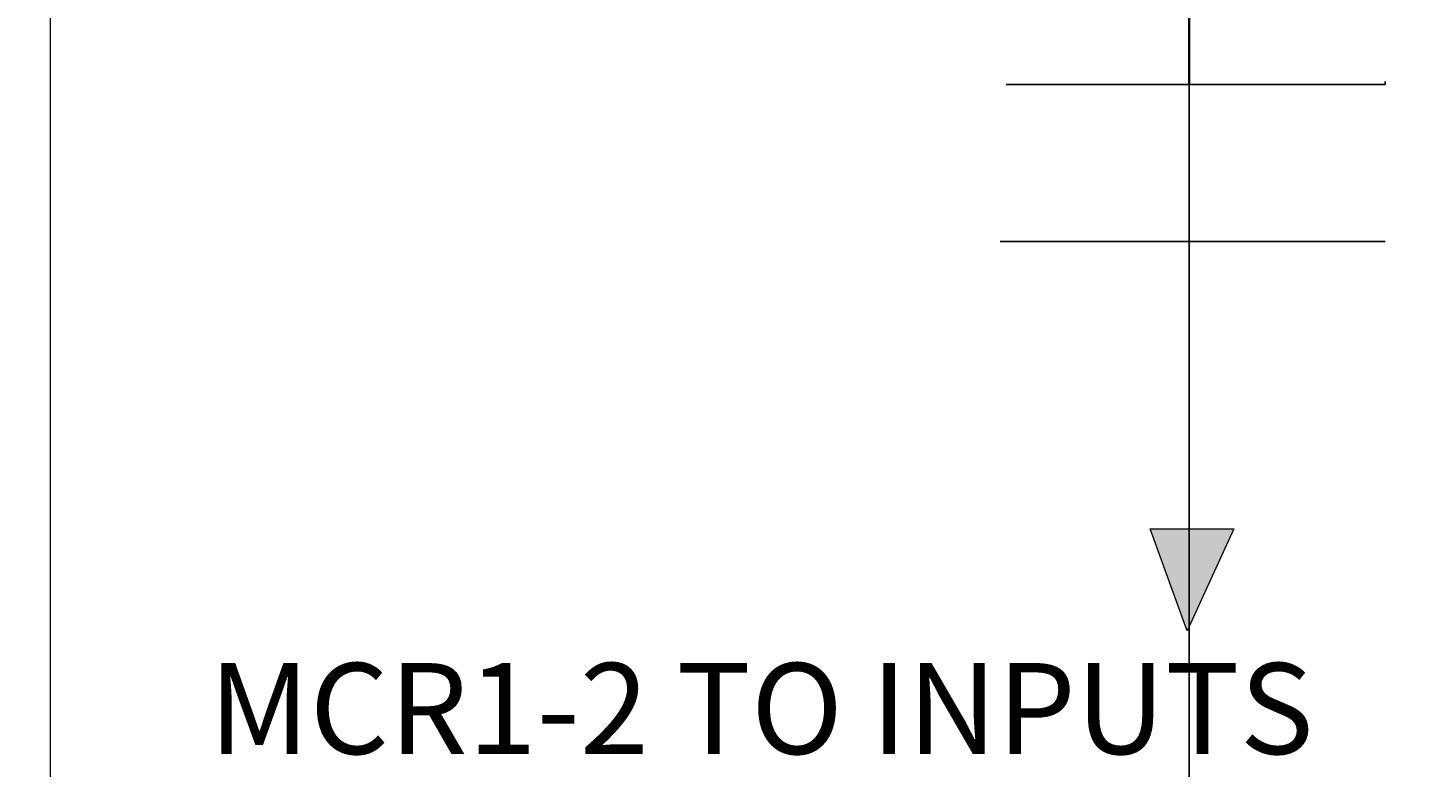
# Model space of a CAD drawing. Units: inches. Extents: x 738 to 1068, y 378 to 757.
# Tile 5 of 41: x 756 to 787, y 416 to 433. Entities that reach past the tile are written whole.
import ezdxf

# ---------------------------------------------------------------- set-up
doc = ezdxf.new("R2010")
doc.units = ezdxf.units.IN
doc.header["$MEASUREMENT"] = 0
for name, color, linetype, lineweight in [('A-ANNO-DIMS', 2, 'Continuous', 18), ('E-ANNO-SYMB', 7, 'Continuous', 18), ('E-ANNO-TEXT', 7, 'Continuous', 18), ('E-CTRL-CONT', 4, 'Continuous', 25), ('E-CTRL-WIRE', 7, 'Continuous', 18), ('E-POWR-FEED', 7, 'Continuous', 35)]:
    doc.layers.add(name, color=color, linetype=linetype, lineweight=lineweight)
doc.styles.get("Standard").update_dxf_attribs({"font": 'arial.ttf'})
doc.dimstyles.get("Standard").update_dxf_attribs({"dimtxt": 0.18, "dimasz": 0.18, "dimexe": 0.18, "dimexo": 0.0625, "dimgap": 0.09, "dimtad": 0, "dimtih": 1, "dimtoh": 1, "dimdec": 4, "dimzin": 0, "dimdsep": 46, "dimtxsty": 'Standard', "dimcen": 0.09, "dimadec": 0, "dimazin": 0, "dimtfac": 1, "dimtdec": 4, "dimtofl": 0, "dimtmove": 0, "dimatfit": 3, "dimfxl": 1, "dimtolj": 1, "dimtzin": 0, "dimarcsym": 0})

# ---------------------------------------------------------------- blocks, each defined once
blk = doc.blocks.new('MCR-IO-CONTACT-NO')
for p, q in [((0.136, 3.468), (8.506, 3.468)), ((8.506, 3.468), (8.506, 3.536)), ((0, 0), (8.506, 0))]:
    blk.add_line(p, q)
blk = doc.blocks.new('FEED-CONTINUATION-ARROW')
h = blk.add_hatch(color=256)
h.dxf.hatch_style = 1
h.paths.add_polyline_path([(1.844, 2.252), (0, 2.252), (0.819, 0)])
for p, q in [((0, 2.252), (1.844, 2.252)), ((0.819, 0), (0, 2.252)), ((1.844, 2.252), (0.819, 0))]:
    blk.add_line(p, q)
blk = doc.blocks.new('*D19')
at = {"layer": 'A-ANNO-DIMS', "color": 0, "lineweight": -2, "transparency": 16777216}
for p, q in [((781.422, 446.265), (738.194, 446.265)), ((738.374, 446.085), (738.374, 421.499)), ((738.374, 396.549), (738.374, 421.135)), ((781.385, 396.369), (738.194, 396.369))]:
    blk.add_line(p, q, dxfattribs=at)
at = {"layer": 'A-ANNO-DIMS', "color": 0, "transparency": 16777216}
for points in [[(738.344, 446.085), (738.404, 446.085), (738.374, 446.265)], [(738.344, 396.549), (738.404, 396.549), (738.374, 396.369)]]:
    blk.add_solid(points, dxfattribs=at)
at = {"layer": 'Defpoints', "color": 0, "transparency": 16777216}
for p in [(738.374, 446.265), (781.485, 446.265), (781.447, 396.369)]:
    blk.add_point(p, dxfattribs=at)
at = {"layer": 'A-ANNO-DIMS', "color": 0, "transparency": 16777216, "insert": (738.374, 421.317), "char_height": 0.18, "attachment_point": 5}
blk.add_mtext('\\A1;49.9', dxfattribs=at)
blk = doc.blocks.new('*D25')
at = {"layer": 'A-ANNO-DIMS', "color": 0, "lineweight": -2, "transparency": 16777216}
for p, q in [((781.49, 646.923), (781.49, 378.239)), ((803.522, 646.923), (803.522, 378.239)), ((781.67, 378.419), (792.111, 378.419)), ((803.342, 378.419), (792.901, 378.419))]:
    blk.add_line(p, q, dxfattribs=at)
at = {"layer": 'A-ANNO-DIMS', "color": 0, "transparency": 16777216}
for points in [[(781.67, 378.449), (781.67, 378.389), (781.49, 378.419)], [(803.342, 378.449), (803.342, 378.389), (803.522, 378.419)]]:
    blk.add_solid(points, dxfattribs=at)
at = {"layer": 'Defpoints', "color": 0, "transparency": 16777216}
for p in [(781.49, 646.985), (803.522, 646.985), (803.522, 378.419)]:
    blk.add_point(p, dxfattribs=at)
at = {"layer": 'A-ANNO-DIMS', "color": 0, "transparency": 16777216, "insert": (792.506, 378.419), "char_height": 0.18, "attachment_point": 5}
blk.add_mtext('\\A1;22.03', dxfattribs=at)
blk = doc.blocks.new('*D34')
at = {"layer": 'A-ANNO-DIMS', "color": 0, "lineweight": -2, "transparency": 16777216}
for p, q in [((781.49, 686.266), (781.49, 378.239)), ((830.489, 686.266), (830.489, 378.239)), ((781.67, 378.419), (805.767, 378.419)), ((830.309, 378.419), (806.212, 378.419))]:
    blk.add_line(p, q, dxfattribs=at)
at = {"layer": 'A-ANNO-DIMS', "color": 0, "transparency": 16777216}
for points in [[(781.67, 378.449), (781.67, 378.389), (781.49, 378.419)], [(830.309, 378.449), (830.309, 378.389), (830.489, 378.419)]]:
    blk.add_solid(points, dxfattribs=at)
at = {"layer": 'Defpoints', "color": 0, "transparency": 16777216}
for p in [(781.49, 686.329), (830.489, 686.329), (830.489, 378.419)]:
    blk.add_point(p, dxfattribs=at)
at = {"layer": 'A-ANNO-DIMS', "color": 0, "transparency": 16777216, "insert": (805.99, 378.419), "char_height": 0.18, "attachment_point": 5}
blk.add_mtext('\\A1;49', dxfattribs=at)
blk = doc.blocks.new('*D38')
at = {"layer": 'A-ANNO-DIMS', "color": 0, "lineweight": -2, "transparency": 16777216}
for p, q in [((781.485, 593.017), (781.485, 378.239)), ((887.04, 593.067), (887.04, 378.239)), ((781.665, 378.419), (833.807, 378.419)), ((886.86, 378.419), (834.718, 378.419))]:
    blk.add_line(p, q, dxfattribs=at)
at = {"layer": 'A-ANNO-DIMS', "color": 0, "transparency": 16777216}
for points in [[(781.665, 378.449), (781.665, 378.389), (781.485, 378.419)], [(886.86, 378.449), (886.86, 378.389), (887.04, 378.419)]]:
    blk.add_solid(points, dxfattribs=at)
at = {"layer": 'Defpoints', "color": 0, "transparency": 16777216}
for p in [(781.485, 593.08), (887.04, 593.13), (887.04, 378.419)]:
    blk.add_point(p, dxfattribs=at)
at = {"layer": 'A-ANNO-DIMS', "color": 0, "transparency": 16777216, "insert": (834.263, 378.419), "char_height": 0.18, "attachment_point": 5}
blk.add_mtext('\\A1;105.56', dxfattribs=at)

msp = doc.modelspace()

# ---------------------------------------------------------------- linework, layer by layer
at = {"layer": 'E-CTRL-WIRE'}
for p, q in [((756.3236, 446.2651), (756.3236, 415.904)), ((781.4897, 427.853), (781.4897, 421.5166))]:
    msp.add_line(p, q, dxfattribs=at)
at = {"layer": 'E-POWR-FEED'}
msp.add_line((781.4897, 437.8486), (781.4897, 431.3208), dxfattribs=at)

# ---------------------------------------------------------------- block references
at = {"layer": 'E-ANNO-SYMB'}
msp.add_blockref('FEED-CONTINUATION-ARROW', (780.628, 419.247), dxfattribs=at)
at = {"layer": 'E-CTRL-CONT'}
msp.add_blockref('MCR-IO-CONTACT-NO', (777.311, 427.853), dxfattribs=at)

# ---------------------------------------------------------------- texts
at = {"layer": 'E-ANNO-TEXT'}
msp.add_text('MCR1-2 TO INPUTS ', height=2.011039, dxfattribs=at).set_placement((759.8319, 416.5202))

# ---------------------------------------------------------------- dimensions: what is measured, and where the dimension line sits
at = {"layer": 'A-ANNO-DIMS'}
for base, p1, p2, override, picture, middle in [((830.4893, 378.4191), (781.4897, 686.329), (830.4893, 686.329), {"dimdec": 0, "dimlfac": 1, "dimrnd": 0, "dimzin": 0, "dimdsep": 46, "dimlunit": 2}, '*D34', (805.9895, 378.4191)), ((803.5218, 378.4191), (781.4897, 646.9853), (803.5218, 646.9853), {"dimdec": 2, "dimlfac": 1, "dimrnd": 0, "dimzin": 0, "dimdsep": 46, "dimlunit": 2}, '*D25', (792.5057, 378.4191)), ((887.0404, 378.4191), (781.4846, 593.0796), (887.0404, 593.1296), {"dimdec": 2, "dimlfac": 1, "dimrnd": 0, "dimzin": 0, "dimdsep": 46, "dimlunit": 2}, '*D38', (834.2625, 378.4191))]:
    dim = msp.add_linear_dim(base=base, p1=p1, p2=p2, dimstyle='Standard', override=override, dxfattribs=at)
    dim.commit()
    dim.dimension.update_dxf_attribs({"geometry": picture, "text_midpoint": middle})
dim = msp.add_linear_dim(base=(738.3736, 446.2651), p1=(781.4474, 396.3691), p2=(781.4846, 446.2651), angle=90, dimstyle='Standard', override={"dimdec": 1, "dimlfac": 1, "dimrnd": 0, "dimzin": 0, "dimdsep": 46, "dimlunit": 2}, dxfattribs=at)
dim.commit()
dim.dimension.update_dxf_attribs({"geometry": '*D19', "text_midpoint": (738.3736, 421.3171)})

doc.saveas('drawing.dxf')
